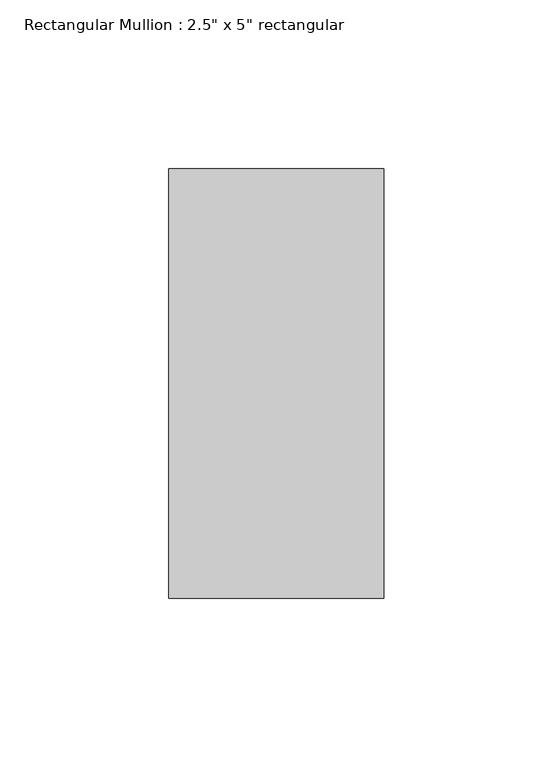
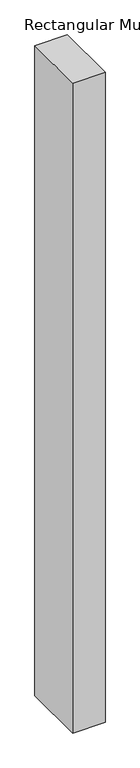
"""IFC4 building model written with IfcOpenShell, lengths in millimetres: member geometry."""

from ifc_helpers import new_model, si_unit, frame, origin, place, context, project, spatial, polyline, outline, extrude, source, transform, mapped, element, save


def member_64ac20db(model_context):
    return source(origin(), model_context, "Body", "SweptSolid", [
        extrude(outline(polyline([(31.75, 63.5), (31.75, -63.5), (-31.75, -63.5), (-31.75, 63.5), (31.75, 63.5)])), frame((0.0, 0.0, -1339.8500001), z_axis=(0.0, 0.0, 1.0), x_axis=(1.0, 0.0, 0.0)), (0.0, 0.0, 1.0), 1339.8500001),
    ])


if __name__ == "__main__":
    model = new_model("IFC4")
    model_context = context("Model", 3, world=origin())
    ifc_project = project(units=[si_unit("LENGTHUNIT", "METRE", prefix="MILLI")], contexts=[model_context])
    site = spatial("IfcSite", under=ifc_project)
    building = spatial("IfcBuilding", under=site)
    placement = place(None, origin())
    member_shape = member_64ac20db(model_context)
    element("IfcMember", 1, ObjectType="Rectangular Mullion : 2.5\" x 5\" rectangular", at=placement, inside=building, context=model_context, shape_type="MappedRepresentation", body=[
        mapped(member_shape, transform((0.0, 0.0, 0.0), x_axis=(1.0, 0.0, 0.0), y_axis=(0.0, 1.0, 0.0), z_axis=(0.0, 0.0, 1.0))),
    ])
    save(model, "model.ifc")

# Revit data of these elements
# Type "Rectangular Mullion : 2.5\" x 5\" rectangular"
#   built-in parameter 1007304 = 0.416667 (stored number, unit not read)
#   built-in parameter 1007301 = 0.104167 (stored number, unit not read)
#   built-in parameter 1007300 = 0.104167 (stored number, unit not read)
# Element 1 (IfcMember, "Rectangular Mullion : 2.5\" x 5\" rectangular")
#   Materials on its faces: "Aluminum"
# Materials
#   "Aluminum": class "Metal", colour RGB 247 247 247, transparency 0, Description = "Aluminum 6061", Cost = 0
